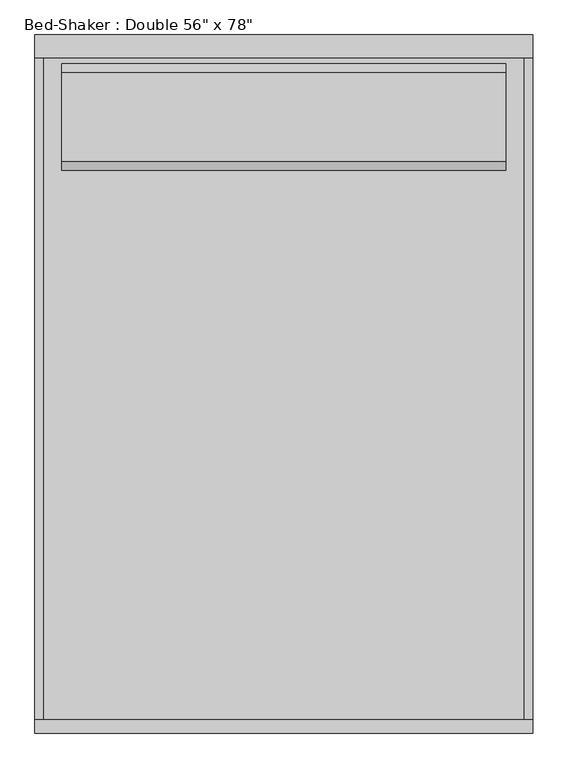
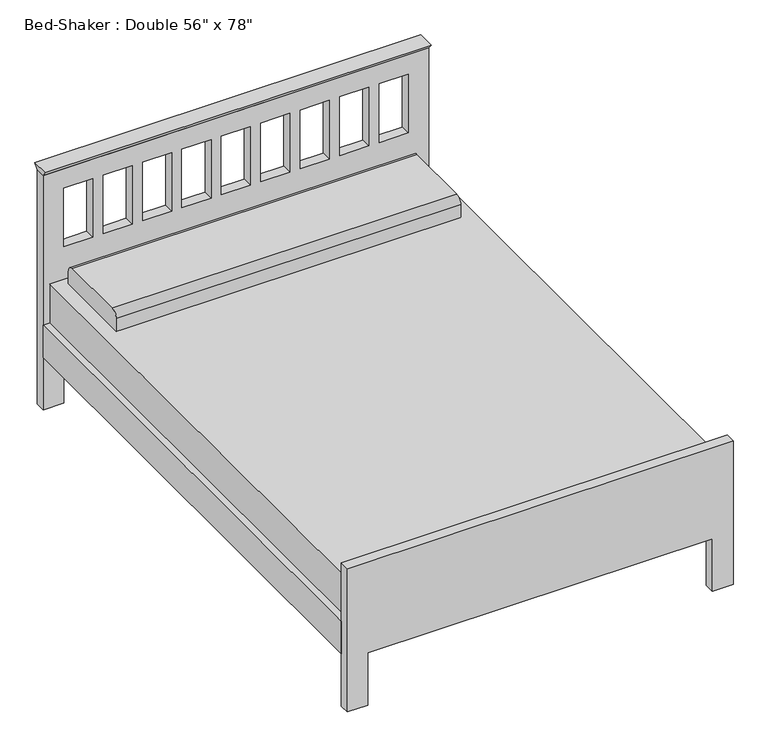
"""IFC4 building model written with IfcOpenShell, lengths in millimetres: furniture geometry."""

from ifc_helpers import new_model, si_unit, point, frame, frame_2d, origin, place, context, project, spatial, polyline, circle_curve, trimmed, segment, composite_curve, outline, extrude, source, transform, mapped, element, save


def furniture_096e7f55(model_context):
    return source(origin(), model_context, "Body", "SweptSolid", [
        extrude(outline(polyline([(-38.1, 914.4), (-51.9545455, 933.45), (13.8545455, 933.45), (0.0, 914.4), (-38.1, 914.4)])), frame((-730.0365546, 0.0, 0.0), z_axis=(1.0, 0.0, 0.0), x_axis=(0.0, 1.0, 0.0)), (0.0, 0.0, 1.0), 1422.4533613),
        extrude(outline(composite_curve([segment(polyline([(-373.2486637, 482.6), (-373.2486637, 533.4)]), True, "CONTINUOUS"), segment(trimmed(circle_curve(frame_2d((-347.8486637, 533.4)), 25.4), [point((-373.2486637, 533.4))], [point((-347.8486637, 558.8))], False, "CARTESIAN"), True, "CONTINUOUS"), segment(polyline([(-347.8486637, 558.8), (-93.8486637, 558.8)]), True, "CONTINUOUS"), segment(trimmed(circle_curve(frame_2d((-93.8486637, 533.4)), 25.4), [point((-93.8486637, 558.8))], [point((-68.4486637, 533.4))], False, "CARTESIAN"), True, "CONTINUOUS"), segment(polyline([(-68.4486637, 533.4), (-68.4486637, 482.6), (-373.2486637, 482.6)]), True, "CONTINUOUS")], self_intersect=False)), frame((-654.05, 0.0, 0.0), z_axis=(1.0, 0.0, 0.0), x_axis=(0.0, 1.0, 0.0)), (0.0, 0.0, 1.0), 1270.0),
        extrude(outline(polyline([(666.75, -38.1), (666.75, -1943.1), (-704.85, -1943.1), (-704.85, -38.1), (666.75, -38.1)])), frame((0.0, 0.0, 228.6), z_axis=(0.0, 0.0, 1.0), x_axis=(1.0, 0.0, 0.0)), (0.0, 0.0, 1.0), 254.0),
        extrude(outline(polyline([(666.75, -1943.1), (666.75, -38.1), (692.15, -38.1), (692.15, -1943.1), (666.75, -1943.1)])), frame((0.0, 0.0, 203.0994861), z_axis=(0.0, 0.0, 1.0), x_axis=(1.0, 0.0, 0.0)), (0.0, 0.0, 1.0), 127.0),
        extrude(outline(polyline([(-730.25, -1943.1), (-730.25, -38.1), (-704.85, -38.1), (-704.85, -1943.1), (-730.25, -1943.1)])), frame((0.0, 0.0, 203.5755296), z_axis=(0.0, 0.0, 1.0), x_axis=(1.0, 0.0, 0.0)), (0.0, 0.0, 1.0), 127.0),
        extrude(outline(polyline([(0.0, -654.05), (203.2, -654.05), (203.2, 615.95), (0.0, 615.95), (0.0, 692.15), (558.8, 692.15), (558.8, -730.25), (0.0, -730.25), (0.0, -654.05)])), frame((0.0, -1981.2, 0.0), z_axis=(0.0, 1.0, 0.0), x_axis=(0.0, 0.0, 1.0)), (0.0, 0.0, 1.0), 38.1),
        extrude(outline(polyline([(914.4, 692.4168067), (914.4, -730.0365546), (0.0, -730.0365546), (0.0, -654.05), (203.2, -654.05), (203.2, 615.95), (0.0, 615.95), (0.0, 692.4168067), (914.4, 692.4168067)]), holes=[polyline([(838.2, -546.8055556), (609.6, -546.8055556), (609.6, -654.05), (838.2, -654.05), (838.2, -546.8055556)]), polyline([(838.2, -401.4611111), (609.6, -401.4611111), (609.6, -508.7055556), (838.2, -508.7055556), (838.2, -401.4611111)]), polyline([(838.2, -256.1166667), (609.6, -256.1166667), (609.6, -363.3611111), (838.2, -363.3611111), (838.2, -256.1166667)]), polyline([(838.2, -110.7722222), (609.6, -110.7722222), (609.6, -218.0166667), (838.2, -218.0166667), (838.2, -110.7722222)]), polyline([(838.2, 179.9166667), (609.6, 179.9166667), (609.6, 72.6722222), (838.2, 72.6722222), (838.2, 179.9166667)]), polyline([(838.2, 325.2611111), (609.6, 325.2611111), (609.6, 218.0166667), (838.2, 218.0166667), (838.2, 325.2611111)]), polyline([(838.2, 470.6055556), (609.6, 470.6055556), (609.6, 363.3611111), (838.2, 363.3611111), (838.2, 470.6055556)]), polyline([(838.2, 615.95), (609.6, 615.95), (609.6, 508.7055556), (838.2, 508.7055556), (838.2, 615.95)]), polyline([(838.2, 34.5722222), (609.6, 34.5722222), (609.6, -72.6722222), (838.2, -72.6722222), (838.2, 34.5722222)])]), frame((0.0, -38.1, 0.0), z_axis=(0.0, 1.0, 0.0), x_axis=(0.0, 0.0, 1.0)), (0.0, 0.0, 1.0), 38.1),
    ])


if __name__ == "__main__":
    model = new_model("IFC4")
    model_context = context("Model", 3, world=origin())
    ifc_project = project(units=[si_unit("LENGTHUNIT", "METRE", prefix="MILLI")], contexts=[model_context])
    site = spatial("IfcSite", under=ifc_project)
    building = spatial("IfcBuilding", under=site)
    placement = place(None, origin())
    furniture_shape = furniture_096e7f55(model_context)
    element("IfcFurniture", 1, ObjectType="Bed-Shaker : Double 56\" x 78\"", at=placement, inside=building, context=model_context, shape_type="MappedRepresentation", body=[
        mapped(furniture_shape, transform((0.0, 0.0, 0.0), x_axis=(1.0, 0.0, 0.0), y_axis=(0.0, 1.0, 0.0), z_axis=(0.0, 0.0, 1.0))),
    ])
    save(model, "model.ifc")

# Revit data of these elements
# Type "Bed-Shaker : Double 56\" x 78\""
#   Assembly Code = "E2020200"
#   Length = 6' - 6"
#   Width = 4' - 8"
#   Frame Material = Birch
#   Mattress Material = Sash
#   Default Elevation = 0
# Element 1 (IfcFurniture, "Bed-Shaker : Double 56\" x 78\"")
#   Materials on its faces: "Birch", "Sash"
# Materials
#   "Birch": class "Wood", colour RGB 224 178 126, transparency 0, Description = "Betula Alleghaniensis", Cost = 0
#   "Sash": class "Wood", colour RGB 224 178 126, transparency 0
